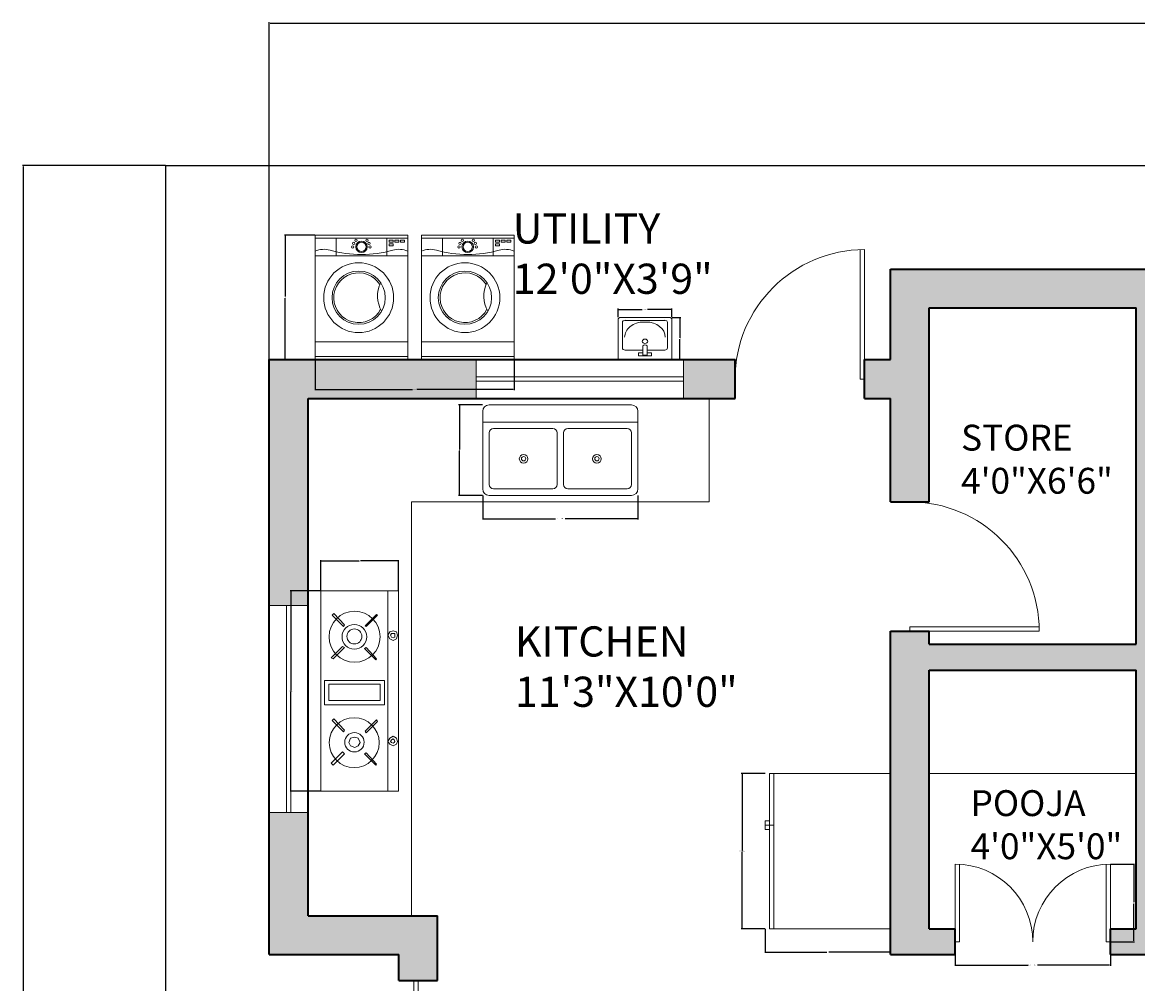
# Model space of a CAD drawing. Units: inches. Extents: x 3386 to 4477, y 1118 to 1824.
# Tile 3 of 7: x 3386 to 3645, y 1601 to 1824. Entities that reach past the tile are written whole.
import ezdxf

# ---------------------------------------------------------------- set-up
doc = ezdxf.new("R2010")
doc.units = ezdxf.units.IN
for name, color, linetype, lineweight in [('A-ANNO-DIMS', 2, 'Continuous', 18), ('A-AREA-IDEN', 7, 'Continuous', 18), ('A-DOOR', 4, 'Continuous', 18), ('A-EQPM', 9, 'Continuous', 18), ('A-FLOR-CASE', 7, 'Continuous', 18), ('A-GLAZ', 4, 'Continuous', 18), ('A-WALL', 7, 'Continuous', 35), ('C-PROP', 7, 'Continuous', 25), ('Сантехника', 7, 'Continuous', 18)]:
    doc.layers.add(name, color=color, linetype=linetype, lineweight=lineweight)
doc.layers.add('A-WALL-PATT', color=18, linetype='Continuous', lineweight=13, true_color=0x000000)
doc.styles.get("Standard").update_dxf_attribs({"font": 'arial.ttf'})
doc.dimstyles.get("Standard").update_dxf_attribs({"dimtxt": 0.18, "dimasz": 0.18, "dimexe": 0.18, "dimexo": 0.0625, "dimgap": 0.09, "dimtad": 0, "dimtih": 1, "dimtoh": 1, "dimdec": 4, "dimzin": 0, "dimdsep": 46, "dimtxsty": 'Standard', "dimcen": 0.09, "dimadec": 0, "dimazin": 0, "dimtfac": 1, "dimtdec": 4, "dimtofl": 0, "dimtmove": 0, "dimatfit": 3, "dimfxl": 1, "dimtolj": 1, "dimtzin": 0, "dimarcsym": 0})

# ---------------------------------------------------------------- blocks, each defined once
blk = doc.blocks.new('D2')
for p, q in [((0, 30), (0, 0)), ((1, 30), (1, 0)), ((0, 0), (1, 0))]:
    blk.add_line(p, q)
blk.add_arc((0, 0), 30, 0, 90)
blk = doc.blocks.new('D3')
for p, q in [((0, 0), (0, 18)), ((1, 0), (1, 18)), ((35, 0), (35, 18)), ((36, 0), (36, 18)), ((0, 0), (1, 0)), ((36, 0), (35, 0))]:
    blk.add_line(p, q)
for centre, start, end in [((0, 0), 0, 90), ((36, 0), 90, 180)]:
    blk.add_arc(centre, 18, start, end)
blk = doc.blocks.new('wash')
at = {"layer": 'Сантехника'}
for p, q in [((4817.13, 2840.92), (4788.24, 2840.92)), ((4788.24, 2819.46), (4788.24, 2840.92)), ((4788.93, 2819.46), (4788.93, 2840.92)), ((4793.08, 2819.46), (4793.08, 2840.92)), ((4812.98, 2819.46), (4812.98, 2840.92)), ((4816.44, 2819.46), (4816.44, 2840.92)), ((4817.13, 2819.46), (4817.13, 2840.92)), ((4793.08, 2836.07), (4788.93, 2836.07)), ((4793.08, 2824.31), (4788.93, 2824.31)), ((4817.13, 2819.46), (4788.24, 2819.46)), ((4817.13, 2816.27), (4788.24, 2816.27)), ((4788.24, 2794.82), (4788.24, 2816.27)), ((4788.93, 2794.82), (4788.93, 2816.27)), ((4793.08, 2794.82), (4793.08, 2816.27)), ((4812.98, 2794.82), (4812.98, 2816.27)), ((4816.44, 2794.82), (4816.44, 2816.27)), ((4817.13, 2794.82), (4817.13, 2816.27)), ((4793.08, 2811.43), (4788.93, 2811.43)), ((4793.08, 2799.66), (4788.93, 2799.66)), ((4817.13, 2794.82), (4788.24, 2794.82))]:
    blk.add_line(p, q, dxfattribs=at)
for points in [[(4789.4, 2839.27), (4789.4, 2840.17), (4789.9, 2840.17), (4789.9, 2839.27)], [(4789.4, 2837.95), (4789.4, 2838.85), (4789.9, 2838.85), (4789.9, 2837.95)], [(4789.4, 2836.64), (4789.4, 2837.53), (4789.9, 2837.53), (4789.9, 2836.64)], [(4790.27, 2836.64), (4790.27, 2837.53), (4790.77, 2837.53), (4790.77, 2836.64)], [(4789.4, 2814.62), (4789.4, 2815.52), (4789.9, 2815.52), (4789.9, 2814.62)], [(4789.4, 2813.31), (4789.4, 2814.2), (4789.9, 2814.2), (4789.9, 2813.31)], [(4789.4, 2811.99), (4789.4, 2812.89), (4789.9, 2812.89), (4789.9, 2811.99)], [(4790.27, 2811.99), (4790.27, 2812.89), (4790.77, 2812.89), (4790.77, 2811.99)]]:
    blk.add_lwpolyline(points, close=True, dxfattribs=at)
for centre, radius in [((4802.77, 2829.54), 8.1), ((4802.77, 2829.54), 6.17), ((4789.46, 2831.45), 0.271), ((4790.19, 2831.93), 0.271), ((4790.98, 2832.18), 0.271), ((4789.46, 2828.92), 0.271), ((4790.98, 2830.19), 1.34), ((4790.98, 2830.19), 1.07), ((4790.19, 2828.4), 0.271), ((4790.98, 2828.15), 0.271), ((4802.77, 2804.9), 8.1), ((4802.77, 2804.9), 6.17), ((4789.46, 2806.8), 0.271), ((4790.98, 2805.55), 1.34), ((4790.19, 2807.28), 0.271), ((4790.98, 2805.55), 1.07), ((4790.98, 2807.53), 0.271), ((4789.46, 2804.27), 0.271), ((4790.19, 2803.75), 0.271), ((4790.98, 2803.5), 0.271)]:
    blk.add_circle(centre, radius, dxfattribs=at)
for centre, radius, start, end in [((4796.44, 2838.85), 4.89, 154.895, 196.6068), ((4762.87, 2829.66), 29.92, 1.0206, 15.0937), ((4802.77, 2829.54), 5.77, 121.8067, 62.1506), ((4802.39, 2840.74), 6.83, 243.19, 300.7673), ((4762.87, 2830.72), 29.92, 344.9063, 358.9794), ((4796.44, 2821.54), 4.89, 163.3932, 205.105), ((4796.44, 2814.2), 4.89, 154.895, 196.6068), ((4762.87, 2805.01), 29.92, 1.0206, 15.0937), ((4802.77, 2804.9), 5.77, 121.8067, 62.1506), ((4802.39, 2816.1), 6.83, 243.19, 300.7673), ((4762.87, 2806.08), 29.92, 344.9063, 358.9794), ((4796.44, 2796.89), 4.89, 163.3932, 205.105)]:
    blk.add_arc(centre, radius, start, end, dxfattribs=at)
blk = doc.blocks.new('Rac7')
at = {"color": 0}
for p, q in [((-39501, -24232), (-39501, -23830)), ((-39474, -23808), (-38988, -23808)), ((-38961, -23830), (-38961, -24232)), ((-39457, -23859), (-39457, -24115)), ((-39032, -23838), (-39430, -23838)), ((-39221, -23855), (-39241, -23855)), ((-39005, -24115), (-39005, -23859)), ((-39005, -23859), (-39005, -23859)), ((-39430, -24136), (-39253, -24136)), ((-39297, -24164), (-39253, -24164)), ((-39297, -24194), (-39297, -24164)), ((-39253, -24186), (-39253, -24094)), ((-39209, -24186), (-39209, -24094)), ((-39209, -24136), (-39032, -24136)), ((-39209, -24164), (-39165, -24164)), ((-39165, -24164), (-39165, -24194)), ((-38961, -24232), (-39501, -24232)), ((-39165, -24194), (-39297, -24194)), ((-39253, -24186), (-39209, -24186))]:
    blk.add_line(p, q, dxfattribs=at)
at = {"color": 0, "extrusion": (0, 0, -1)}
for centre, major_axis, start_param, end_param in [((-39474, -23830), (-27, 0), 0, 1.570796), ((-38988, -23830), (-27, 0), 1.570796, 3.141593), ((-39430, -23859), (-27, 0), 0, 1.570796), ((-39241, -24007), (-194, 0), 0, 1.570796), ((-39221, -24007), (-194, 0), 1.570796, 3.141593), ((-39032, -23859), (-27, 0), 1.570796, 3.141593), ((-39430, -24115), (-27, 0), -1.570796, 0), ((-39231, -24104), (-25.3, 0), 0.552816, 2.588777), ((-39032, -24115), (-27, 0), -3.141593, -1.570796)]:
    blk.add_ellipse(centre, major_axis=major_axis, ratio=0.785714, start_param=start_param, end_param=end_param, dxfattribs=at)
blk.add_ellipse((-39231, -24048), major_axis=(-27.9, 0), ratio=0.785714, dxfattribs=at)
blk = doc.blocks.new('Sink-double - 36 in top')
for p, q in [((-18, -4), (18, -4)), ((-0.75, -18.5), (-0.75, -6.5)), ((0.75, -6.5), (0.75, -18.5))]:
    blk.add_line(p, q)
for points in [[(-16.5, 0), (16.5, 0)], [(-18, -19.5), (-18, -1.5)], [(18, -1.5), (18, -19.5)], [(-16.5, -18.5), (-16.5, -6.5)], [(-15.5, -5.5), (-1.75, -5.5)], [(1.75, -5.5), (15.5, -5.5)], [(16.5, -6.5), (16.5, -18.5)], [(-1.75, -19.5), (-15.5, -19.5)], [(15.5, -19.5), (1.75, -19.5)], [(16.5, -21), (-16.5, -21)]]:
    blk.add_lwpolyline(points)
for centre, radius in [((-8.5, -12.5), 1), ((-8.5, -12.5), 0.5), ((8.5, -12.5), 1), ((8.5, -12.5), 0.5)]:
    blk.add_circle(centre, radius)
for centre, radius, start, end in [((-16.5, -1.5), 1.5, 90, 180), ((16.5, -1.5), 1.5, 0, 90), ((-15.5, -6.5), 1, 90, 180), ((-1.75, -6.5), 1, 0, 90), ((1.75, -6.5), 1, 90, 180), ((15.5, -6.5), 1, 0, 90), ((-16.5, -19.5), 1.5, 180, 270), ((-15.5, -18.5), 1, 180, 270), ((-1.75, -18.5), 1, 270, 0), ((1.75, -18.5), 1, 180, 270), ((15.5, -18.5), 1, 270, 0), ((16.5, -19.5), 1.5, 270, 0)]:
    blk.add_arc(centre, radius, start, end)
blk = doc.blocks.new('gas 1')
for points in [[(35.93, -1.87), (35.93, 0), (0, 0), (0, -1.87)], [(8.12, -0.94), (8.44, -1.56), (8.91, -1.87), (9.53, -1.56), (9.84, -0.94), (9.53, -0.31), (8.91, -0.16), (8.44, -0.31)], [(8.59, -0.94), (8.75, -1.25), (8.91, -1.41), (9.22, -1.25), (9.37, -0.94), (9.22, -0.78), (8.91, -0.62), (8.75, -0.78)], [(27.03, -0.94), (27.34, -1.56), (27.97, -1.87), (28.59, -1.56), (28.75, -0.94), (28.59, -0.31), (27.97, -0.16), (27.34, -0.31)], [(27.5, -0.94), (27.65, -1.25), (27.97, -1.41), (28.28, -1.25), (28.28, -0.94), (28.28, -0.62), (27.97, -0.62), (27.65, -0.62)], [(4.84, -3.91), (4.69, -4.06), (6.72, -6.09), (6.87, -5.78)], [(12.81, -3.91), (12.5, -3.75), (10.47, -5.78), (10.78, -5.94)], [(19.84, -13.28), (15.47, -13.28), (15.47, -2.5), (19.84, -2.5)], [(19.22, -12.5), (16.25, -12.5), (16.25, -3.28), (19.22, -3.28)], [(23.75, -3.91), (23.59, -4.06), (25.62, -6.09), (25.78, -5.78)], [(31.71, -3.91), (31.56, -3.75), (29.53, -5.78), (29.68, -5.94)], [(7.81, -7.81), (8.12, -8.59), (8.75, -8.91), (9.53, -8.59), (9.69, -7.81), (9.53, -7.19), (8.75, -6.87), (8.12, -7.19)], [(7.03, -10), (6.72, -9.69), (4.69, -11.72), (5, -12.03)], [(12.97, -11.56), (10.94, -9.69), (10.62, -9.84), (12.65, -11.87)], [(23.75, -11.72), (23.9, -12.03), (25.93, -10), (25.78, -9.69)], [(31.87, -11.56), (29.84, -9.69), (29.53, -9.84), (31.56, -11.87)]]:
    blk.add_lwpolyline(points, close=True)
blk.add_lwpolyline([(35.93, -1.87), (35.93, -13.9), (0, -13.9), (0, -1.87)])
for centre, radius in [((8.7, -7.92), 4.48), ((27.7, -7.86), 4.58), ((27.69, -7.89), 2.22), ((8.77, -7.89), 1.74), ((27.76, -7.89), 1.35)]:
    blk.add_circle(centre, radius)
blk = doc.blocks.new('Refrigerator-2 door - 36 in top')
for p, q in [((0, -26.999999), (36, -26.999999)), ((11, -27.999999), (11, -28.999999)), ((12, -26.999999), (12, -28.999999)), ((13, -28.999999), (13, -27.999999)), ((11, -28.999999), (13, -28.999999))]:
    blk.add_line(p, q)
blk.add_lwpolyline([(0, -27.999999), (0, 0), (36, 0), (36, -27.999999)], close=True)
blk = doc.blocks.new('WIN-48IN')
for p, q in [((0, 48), (9, 48)), ((4, 0), (4, 48)), ((5, 0), (5, 48)), ((0, 0), (9, 0))]:
    blk.add_line(p, q)
blk = doc.blocks.new('DOOR-SLIDING-84IN')
for p, q in [((0, 42), (0, 84)), ((1, 84), (1, 0)), ((1, 42), (0, 42)), ((1, 42), (2, 42)), ((2, 42), (2, 0))]:
    blk.add_line(p, q)
blk = doc.blocks.new('*D69')
at = {"layer": 'A-ANNO-DIMS', "color": 0, "lineweight": -2, "transparency": 16777216}
for p, q in [((3602.66, 1610.81), (3602.66, 1605.29)), ((3638.66, 1610.81), (3638.66, 1605.29)), ((3602.84, 1605.47), (3619.57, 1605.47)), ((3638.48, 1605.47), (3621.74, 1605.47))]:
    blk.add_line(p, q, dxfattribs=at)
at = {"layer": 'A-ANNO-DIMS', "color": 0, "transparency": 16777216}
for points in [[(3602.84, 1605.5), (3602.84, 1605.44), (3602.66, 1605.47)], [(3638.48, 1605.5), (3638.48, 1605.44), (3638.66, 1605.47)]]:
    blk.add_solid(points, dxfattribs=at)
at = {"layer": 'Defpoints', "color": 0, "transparency": 16777216}
for p in [(3602.66, 1610.87), (3638.66, 1610.87), (3638.66, 1605.47)]:
    blk.add_point(p, dxfattribs=at)
at = {"layer": 'A-ANNO-DIMS', "color": 0, "transparency": 16777216, "insert": (3620.66, 1605.47), "char_height": 0.18, "attachment_point": 5}
blk.add_mtext('\\A1;POOJA DOOR 36', dxfattribs=at)
blk = doc.blocks.new('*D70')
at = {"layer": 'A-ANNO-DIMS', "color": 0, "lineweight": -2, "transparency": 16777216}
for p, q in [((3638.72, 1628.87), (3644.24, 1628.87)), ((3644.06, 1628.69), (3644.06, 1620.05)), ((3644.06, 1611.05), (3644.06, 1619.69)), ((3638.72, 1610.87), (3644.24, 1610.87))]:
    blk.add_line(p, q, dxfattribs=at)
at = {"layer": 'A-ANNO-DIMS', "color": 0, "transparency": 16777216}
for points in [[(3644.03, 1628.69), (3644.09, 1628.69), (3644.06, 1628.87)], [(3644.03, 1611.05), (3644.09, 1611.05), (3644.06, 1610.87)]]:
    blk.add_solid(points, dxfattribs=at)
at = {"layer": 'Defpoints', "color": 0, "transparency": 16777216}
for p in [(3638.66, 1628.87), (3644.06, 1628.87), (3638.66, 1610.87)]:
    blk.add_point(p, dxfattribs=at)
at = {"layer": 'A-ANNO-DIMS', "color": 0, "transparency": 16777216, "insert": (3644.06, 1619.87), "char_height": 0.18, "attachment_point": 5}
blk.add_mtext('\\A1;18', dxfattribs=at)
blk = doc.blocks.new('*D87')
at = {"layer": 'A-ANNO-DIMS', "color": 0, "lineweight": -2, "transparency": 16777216}
for p, q in [((3454.3, 1745.81), (3454.3, 1738.77)), ((3500.4, 1745.81), (3500.4, 1738.77)), ((3454.48, 1738.95), (3476.85, 1738.95)), ((3500.22, 1738.95), (3477.85, 1738.95))]:
    blk.add_line(p, q, dxfattribs=at)
at = {"layer": 'A-ANNO-DIMS', "color": 0, "transparency": 16777216}
for points in [[(3454.48, 1738.98), (3454.48, 1738.92), (3454.3, 1738.95)], [(3500.22, 1738.98), (3500.22, 1738.92), (3500.4, 1738.95)]]:
    blk.add_solid(points, dxfattribs=at)
at = {"layer": 'Defpoints', "color": 0, "transparency": 16777216}
for p in [(3454.3, 1745.87), (3500.4, 1745.87), (3500.4, 1738.95)]:
    blk.add_point(p, dxfattribs=at)
at = {"layer": 'A-ANNO-DIMS', "color": 0, "transparency": 16777216, "insert": (3477.35, 1738.95), "char_height": 0.18, "attachment_point": 5}
blk.add_mtext('\\A1;W/D 46', dxfattribs=at)
blk = doc.blocks.new('*D88')
at = {"layer": 'A-ANNO-DIMS', "color": 0, "lineweight": -2, "transparency": 16777216}
for p, q in [((3454.24, 1774.76), (3447.2, 1774.76)), ((3447.38, 1774.58), (3447.38, 1760.5)), ((3447.38, 1746.05), (3447.38, 1760.13)), ((3454.24, 1745.87), (3447.2, 1745.87))]:
    blk.add_line(p, q, dxfattribs=at)
at = {"layer": 'A-ANNO-DIMS', "color": 0, "transparency": 16777216}
for points in [[(3447.35, 1774.58), (3447.41, 1774.58), (3447.38, 1774.76)], [(3447.35, 1746.05), (3447.41, 1746.05), (3447.38, 1745.87)]]:
    blk.add_solid(points, dxfattribs=at)
at = {"layer": 'Defpoints', "color": 0, "transparency": 16777216}
for p in [(3454.3, 1774.76), (3447.38, 1745.87), (3454.3, 1745.87)]:
    blk.add_point(p, dxfattribs=at)
at = {"layer": 'A-ANNO-DIMS', "color": 0, "transparency": 16777216, "insert": (3447.38, 1760.32), "char_height": 0.18, "attachment_point": 5}
blk.add_mtext('\\A1;29', dxfattribs=at)
blk = doc.blocks.new('*D89')
at = {"layer": 'A-ANNO-DIMS', "color": 0, "lineweight": -2, "transparency": 16777216}
for p, q in [((3524.53, 1755.72), (3524.53, 1757.71)), ((3524.71, 1757.53), (3530.13, 1757.53)), ((3536.81, 1757.53), (3531.38, 1757.53)), ((3536.99, 1755.72), (3536.99, 1757.71))]:
    blk.add_line(p, q, dxfattribs=at)
at = {"layer": 'A-ANNO-DIMS', "color": 0, "transparency": 16777216}
for points in [[(3524.71, 1757.56), (3524.71, 1757.5), (3524.53, 1757.53)], [(3536.81, 1757.56), (3536.81, 1757.5), (3536.99, 1757.53)]]:
    blk.add_solid(points, dxfattribs=at)
at = {"layer": 'Defpoints', "color": 0, "transparency": 16777216}
for p in [(3524.53, 1757.53), (3524.53, 1755.66), (3536.99, 1755.66)]:
    blk.add_point(p, dxfattribs=at)
at = {"layer": 'A-ANNO-DIMS', "color": 0, "transparency": 16777216, "insert": (3530.76, 1757.53), "char_height": 0.18, "attachment_point": 5}
blk.add_mtext('\\A1;BASIN 12', dxfattribs=at)
blk = doc.blocks.new('*D90')
at = {"layer": 'A-ANNO-DIMS', "color": 0, "lineweight": -2, "transparency": 16777216}
for p, q in [((3537.05, 1755.66), (3539.04, 1755.66)), ((3538.86, 1755.48), (3538.86, 1750.95)), ((3538.86, 1746.05), (3538.86, 1750.58)), ((3537.05, 1745.87), (3539.04, 1745.87))]:
    blk.add_line(p, q, dxfattribs=at)
at = {"layer": 'A-ANNO-DIMS', "color": 0, "transparency": 16777216}
for points in [[(3538.83, 1755.48), (3538.89, 1755.48), (3538.86, 1755.66)], [(3538.83, 1746.05), (3538.89, 1746.05), (3538.86, 1745.87)]]:
    blk.add_solid(points, dxfattribs=at)
at = {"layer": 'Defpoints', "color": 0, "transparency": 16777216}
for p in [(3536.99, 1755.66), (3538.86, 1755.66), (3536.99, 1745.87)]:
    blk.add_point(p, dxfattribs=at)
at = {"layer": 'A-ANNO-DIMS', "color": 0, "transparency": 16777216, "insert": (3538.86, 1750.76), "char_height": 0.18, "attachment_point": 5}
blk.add_mtext('\\A1;10', dxfattribs=at)
blk = doc.blocks.new('*D95')
at = {"layer": 'A-ANNO-DIMS', "color": 0, "lineweight": -2, "transparency": 16777216}
for p, q in [((3493.13, 1714.32), (3493.13, 1708.8)), ((3529.13, 1714.32), (3529.13, 1708.8)), ((3493.31, 1708.98), (3510.04, 1708.98)), ((3528.95, 1708.98), (3512.23, 1708.98))]:
    blk.add_line(p, q, dxfattribs=at)
at = {"layer": 'A-ANNO-DIMS', "color": 0, "transparency": 16777216}
for points in [[(3493.31, 1709.01), (3493.31, 1708.95), (3493.13, 1708.98)], [(3528.95, 1709.01), (3528.95, 1708.95), (3529.13, 1708.98)]]:
    blk.add_solid(points, dxfattribs=at)
at = {"layer": 'Defpoints', "color": 0, "transparency": 16777216}
for p in [(3493.13, 1714.38), (3529.13, 1714.38), (3493.13, 1708.98)]:
    blk.add_point(p, dxfattribs=at)
at = {"layer": 'A-ANNO-DIMS', "color": 0, "transparency": 16777216, "insert": (3511.13, 1708.98), "char_height": 0.18, "attachment_point": 5}
blk.add_mtext('\\A1;DOUBLE SINK 36', dxfattribs=at)
blk = doc.blocks.new('*D96')
at = {"layer": 'A-ANNO-DIMS', "color": 0, "lineweight": -2, "transparency": 16777216}
for p, q in [((3493.07, 1735.38), (3487.55, 1735.38)), ((3487.73, 1735.2), (3487.73, 1725.06)), ((3487.73, 1714.56), (3487.73, 1724.7)), ((3493.07, 1714.38), (3487.55, 1714.38))]:
    blk.add_line(p, q, dxfattribs=at)
at = {"layer": 'A-ANNO-DIMS', "color": 0, "transparency": 16777216}
for points in [[(3487.7, 1735.2), (3487.76, 1735.2), (3487.73, 1735.38)], [(3487.7, 1714.56), (3487.76, 1714.56), (3487.73, 1714.38)]]:
    blk.add_solid(points, dxfattribs=at)
at = {"layer": 'Defpoints', "color": 0, "transparency": 16777216}
for p in [(3487.73, 1735.38), (3493.13, 1735.38), (3493.13, 1714.38)]:
    blk.add_point(p, dxfattribs=at)
at = {"layer": 'A-ANNO-DIMS', "color": 0, "transparency": 16777216, "insert": (3487.73, 1724.88), "char_height": 0.18, "attachment_point": 5}
blk.add_mtext('\\A1;21', dxfattribs=at)
blk = doc.blocks.new('*D97')
at = {"layer": 'A-ANNO-DIMS', "color": 0, "lineweight": -2, "transparency": 16777216}
for p, q in [((3455.55, 1692.24), (3448.47, 1692.24)), ((3448.65, 1692.06), (3448.65, 1669.2)), ((3448.65, 1645.97), (3448.65, 1668.83)), ((3455.55, 1645.79), (3448.47, 1645.79))]:
    blk.add_line(p, q, dxfattribs=at)
at = {"layer": 'A-ANNO-DIMS', "color": 0, "transparency": 16777216}
for points in [[(3448.62, 1692.06), (3448.68, 1692.06), (3448.65, 1692.24)], [(3448.62, 1645.97), (3448.68, 1645.97), (3448.65, 1645.79)]]:
    blk.add_solid(points, dxfattribs=at)
at = {"layer": 'Defpoints', "color": 0, "transparency": 16777216}
for p in [(3448.65, 1692.24), (3455.61, 1692.24), (3455.61, 1645.79)]:
    blk.add_point(p, dxfattribs=at)
at = {"layer": 'A-ANNO-DIMS', "color": 0, "transparency": 16777216, "insert": (3448.65, 1669.01), "char_height": 0.18, "attachment_point": 5}
blk.add_mtext('\\A1;HOB 46', dxfattribs=at)
blk = doc.blocks.new('*D98')
at = {"layer": 'A-ANNO-DIMS', "color": 0, "lineweight": -2, "transparency": 16777216}
for p, q in [((3455.61, 1692.3), (3455.61, 1699.38)), ((3455.79, 1699.2), (3464.39, 1699.2)), ((3473.41, 1699.2), (3464.81, 1699.2)), ((3473.59, 1692.3), (3473.59, 1699.38))]:
    blk.add_line(p, q, dxfattribs=at)
at = {"layer": 'A-ANNO-DIMS', "color": 0, "transparency": 16777216}
for points in [[(3455.79, 1699.23), (3455.79, 1699.17), (3455.61, 1699.2)], [(3473.41, 1699.23), (3473.41, 1699.17), (3473.59, 1699.2)]]:
    blk.add_solid(points, dxfattribs=at)
at = {"layer": 'Defpoints', "color": 0, "transparency": 16777216}
for p in [(3473.59, 1699.2), (3455.61, 1692.24), (3473.59, 1692.24)]:
    blk.add_point(p, dxfattribs=at)
at = {"layer": 'A-ANNO-DIMS', "color": 0, "transparency": 16777216, "insert": (3464.6, 1699.2), "char_height": 0.18, "attachment_point": 5}
blk.add_mtext('\\A1;18', dxfattribs=at)
blk = doc.blocks.new('*D99')
at = {"layer": 'A-ANNO-DIMS', "color": 0, "lineweight": -2, "transparency": 16777216}
for p, q in [((3558.59, 1649.87), (3553.08, 1649.87)), ((3553.26, 1649.69), (3553.26, 1632.05)), ((3553.26, 1614.05), (3553.26, 1631.68)), ((3558.59, 1613.87), (3553.08, 1613.87))]:
    blk.add_line(p, q, dxfattribs=at)
at = {"layer": 'A-ANNO-DIMS', "color": 0, "transparency": 16777216}
for points in [[(3553.23, 1649.69), (3553.29, 1649.69), (3553.26, 1649.87)], [(3553.23, 1614.05), (3553.29, 1614.05), (3553.26, 1613.87)]]:
    blk.add_solid(points, dxfattribs=at)
at = {"layer": 'Defpoints', "color": 0, "transparency": 16777216}
for p in [(3558.66, 1649.87), (3553.26, 1613.87), (3558.66, 1613.87)]:
    blk.add_point(p, dxfattribs=at)
at = {"layer": 'A-ANNO-DIMS', "color": 0, "transparency": 16777216, "insert": (3553.26, 1631.87), "char_height": 0.18, "attachment_point": 5}
blk.add_mtext('\\A1;FRIDGE 36', dxfattribs=at)
blk = doc.blocks.new('*D100')
at = {"layer": 'A-ANNO-DIMS', "color": 0, "lineweight": -2, "transparency": 16777216}
for p, q in [((3558.66, 1613.81), (3558.66, 1608.29)), ((3587.66, 1613.81), (3587.66, 1608.29)), ((3558.84, 1608.47), (3572.93, 1608.47)), ((3587.48, 1608.47), (3573.38, 1608.47))]:
    blk.add_line(p, q, dxfattribs=at)
at = {"layer": 'A-ANNO-DIMS', "color": 0, "transparency": 16777216}
for points in [[(3558.84, 1608.5), (3558.84, 1608.44), (3558.66, 1608.47)], [(3587.48, 1608.5), (3587.48, 1608.44), (3587.66, 1608.47)]]:
    blk.add_solid(points, dxfattribs=at)
at = {"layer": 'Defpoints', "color": 0, "transparency": 16777216}
for p in [(3558.66, 1613.87), (3587.66, 1613.87), (3587.66, 1608.47)]:
    blk.add_point(p, dxfattribs=at)
at = {"layer": 'A-ANNO-DIMS', "color": 0, "transparency": 16777216, "insert": (3573.16, 1608.47), "char_height": 0.18, "attachment_point": 5}
blk.add_mtext('\\A1;29', dxfattribs=at)
blk = doc.blocks.new('*D102')
at = {"layer": 'A-ANNO-DIMS', "color": 0, "lineweight": -2, "transparency": 16777216}
for p, q in [((3419.59, 1790.87), (3386.43, 1790.87)), ((3386.61, 1790.69), (3386.61, 1491.05)), ((3386.61, 1191.05), (3386.61, 1490.69)), ((3419.59, 1190.87), (3386.43, 1190.87))]:
    blk.add_line(p, q, dxfattribs=at)
at = {"layer": 'A-ANNO-DIMS', "color": 0, "transparency": 16777216}
for points in [[(3386.58, 1790.69), (3386.64, 1790.69), (3386.61, 1790.87)], [(3386.58, 1191.05), (3386.64, 1191.05), (3386.61, 1190.87)]]:
    blk.add_solid(points, dxfattribs=at)
at = {"layer": 'Defpoints', "color": 0, "transparency": 16777216}
for p in [(3386.61, 1790.87), (3419.66, 1790.87), (3419.66, 1190.87)]:
    blk.add_point(p, dxfattribs=at)
at = {"layer": 'A-ANNO-DIMS', "color": 0, "transparency": 16777216, "insert": (3386.61, 1490.87), "char_height": 0.18, "attachment_point": 5}
blk.add_mtext('\\A1;600', dxfattribs=at)
blk = doc.blocks.new('*D103')
at = {"layer": 'A-ANNO-DIMS', "color": 0, "lineweight": -2, "transparency": 16777216}
for p, q in [((3443.66, 1745.93), (3443.66, 1824.1)), ((3443.84, 1823.92), (3659.36, 1823.92)), ((3875.48, 1823.92), (3659.95, 1823.92)), ((3875.66, 1766.93), (3875.66, 1824.1))]:
    blk.add_line(p, q, dxfattribs=at)
at = {"layer": 'A-ANNO-DIMS', "color": 0, "transparency": 16777216}
for points in [[(3443.84, 1823.95), (3443.84, 1823.89), (3443.66, 1823.92)], [(3875.48, 1823.95), (3875.48, 1823.89), (3875.66, 1823.92)]]:
    blk.add_solid(points, dxfattribs=at)
at = {"layer": 'Defpoints', "color": 0, "transparency": 16777216}
for p in [(3875.66, 1823.92), (3875.66, 1766.87), (3443.66, 1745.87)]:
    blk.add_point(p, dxfattribs=at)
at = {"layer": 'A-ANNO-DIMS', "color": 0, "transparency": 16777216, "insert": (3659.66, 1823.92), "char_height": 0.18, "attachment_point": 5}
blk.add_mtext('\\A1;432', dxfattribs=at)

msp = doc.modelspace()

# ---------------------------------------------------------------- hatches: boundary and pattern name
at = {"layer": 'A-WALL-PATT'}
h = msp.add_hatch(color=256, dxfattribs=at)
h.dxf.hatch_style = 1
h.paths.add_polyline_path([(3443.66, 1221.87), (3452.66, 1221.87), (3452.66, 1301.87), (3458.66, 1301.87), (3458.66, 1310.87), (3452.66, 1310.87), (3452.66, 1328.87), (3443.66, 1328.87)])
h.paths.add_polyline_path([(3506.66, 1310.87), (3506.66, 1306.37), (3506.66, 1301.87), (3530.66, 1301.87), (3530.66, 1310.87)])
h.paths.add_polyline_path([(3653.66, 1301.87), (3653.66, 1382.87), (3662.66, 1382.87), (3662.66, 1391.87), (3653.66, 1391.87), (3653.66, 1529.87), (3659.66, 1529.87), (3659.66, 1535.87), (3644.66, 1535.87), (3644.66, 1310.87), (3602.66, 1310.87), (3602.66, 1301.87)])
h.paths.add_polyline_path([(3452.66, 1406.87), (3443.66, 1406.87), (3443.66, 1376.87), (3452.66, 1376.87), (3452.66, 1388.44)])
h.paths.add_polyline_path([(3452.66, 1478.87), (3452.66, 1502.87), (3478.74, 1502.87), (3482.66, 1502.87), (3482.66, 1504.87), (3482.66, 1517.87), (3473.66, 1517.87), (3473.66, 1511.87), (3443.66, 1511.87), (3443.66, 1478.87)])
h.paths.add_polyline_path([(3773.66, 1391.87), (3710.66, 1391.87), (3710.66, 1382.87), (3773.66, 1382.87)], flags=17)
h.paths.add_polyline_path([(3824.66, 1391.87), (3806.66, 1391.87), (3806.66, 1469.87), (3809.66, 1469.87), (3809.66, 1472.87), (3809.66, 1475.87), (3806.66, 1475.87), (3806.66, 1478.87), (3800.66, 1478.87), (3800.66, 1463.32), (3800.66, 1391.87), (3797.66, 1391.87), (3797.66, 1382.87), (3824.66, 1382.87)], flags=17)
h.paths.add_polyline_path([(3866.66, 1469.87), (3866.66, 1391.87), (3848.66, 1391.87), (3848.66, 1382.87), (3875.66, 1382.87), (3875.66, 1547.87), (3866.66, 1547.87), (3866.66, 1535.87), (3695.66, 1535.87), (3695.66, 1529.87), (3800.66, 1529.87), (3800.66, 1508.87), (3806.66, 1508.87), (3806.66, 1529.87), (3866.66, 1529.87), (3866.66, 1475.87), (3839.66, 1475.87), (3839.66, 1469.87)])
h.paths.add_polyline_path([(3875.66, 1673.87), (3866.66, 1673.87), (3866.66, 1663.37), (3866.66, 1647.44), (3866.66, 1613.87), (3761.66, 1613.87), (3761.66, 1607.87), (3866.66, 1607.87), (3866.66, 1595.87), (3875.66, 1595.87)])
h.paths.add_polyline_path([(3473.66, 1607.87), (3473.66, 1601.87), (3482.66, 1601.87), (3482.66, 1616.87), (3452.66, 1616.87), (3452.66, 1640.87), (3443.66, 1640.87), (3443.66, 1607.87)])
h.paths.add_polyline_path([(3491.66, 1736.87), (3491.66, 1745.87), (3478.95, 1745.87), (3443.66, 1745.87), (3443.66, 1688.87), (3452.66, 1688.87), (3452.66, 1736.87)])
h.paths.add_polyline_path([(3551.66, 1745.87), (3539.66, 1745.87), (3539.66, 1736.87), (3551.66, 1736.87)])
h.paths.add_polyline_path([(3587.66, 1745.87), (3581.66, 1745.87), (3581.66, 1741.37), (3581.66, 1736.87), (3587.66, 1736.87), (3587.66, 1712.87), (3596.66, 1712.87), (3596.66, 1757.87), (3644.66, 1757.87), (3644.66, 1679.87), (3596.66, 1679.87), (3596.66, 1682.87), (3592.16, 1682.87), (3587.66, 1682.87), (3587.66, 1607.87), (3602.66, 1607.87), (3602.66, 1613.87), (3596.66, 1613.87), (3596.66, 1673.87), (3644.66, 1673.87), (3644.66, 1613.87), (3638.66, 1613.87), (3638.66, 1610.87), (3638.66, 1607.87), (3725.66, 1607.87), (3725.66, 1613.87), (3722.66, 1613.87), (3722.66, 1634.87), (3716.66, 1634.87), (3716.66, 1613.87), (3650.66, 1613.87), (3650.66, 1673.87), (3683.66, 1673.87), (3683.66, 1679.87), (3650.66, 1679.87), (3650.66, 1757.87), (3671.66, 1757.87), (3671.66, 1766.87), (3587.66, 1766.87)])
h.paths.add_polyline_path([(3716.66, 1757.87), (3716.66, 1679.87), (3713.66, 1679.87), (3713.66, 1673.87), (3716.66, 1673.87), (3716.66, 1664.87), (3722.66, 1664.87), (3722.66, 1757.87), (3728.66, 1757.87), (3728.66, 1766.87), (3695.66, 1766.87), (3695.66, 1757.87)])
h.paths.add_polyline_path([(3806.66, 1757.87), (3806.66, 1766.87), (3776.66, 1766.87), (3776.66, 1757.87)])
h.paths.add_polyline_path([(3875.66, 1766.87), (3854.66, 1766.87), (3854.66, 1757.87), (3866.66, 1757.87), (3866.66, 1733.87), (3875.66, 1733.87)])

# ---------------------------------------------------------------- linework, layer by layer
at = {"layer": 'A-FLOR-CASE'}
for p, q in [((3545.66, 1736.87), (3545.66, 1712.87)), ((3476.66, 1616.87), (3476.66, 1712.87)), ((3476.66, 1712.87), (3545.66, 1712.87)), ((3596.66, 1649.87), (3644.66, 1649.87))]:
    msp.add_line(p, q, dxfattribs=at)
at = {"layer": 'A-WALL'}
for p, q in [((3587.66, 1766.87), (3875.66, 1766.87)), ((3587.66, 1745.87), (3587.66, 1766.87)), ((3596.66, 1757.87), (3644.66, 1757.87)), ((3596.66, 1712.87), (3596.66, 1757.87)), ((3644.66, 1679.87), (3644.66, 1757.87)), ((3443.66, 1607.87), (3443.66, 1745.87)), ((3443.66, 1745.87), (3551.66, 1745.87)), ((3551.66, 1736.87), (3551.66, 1745.87)), ((3581.66, 1736.87), (3581.66, 1745.87)), ((3581.66, 1745.87), (3587.66, 1745.87)), ((3452.66, 1616.87), (3452.66, 1736.87)), ((3452.66, 1736.87), (3551.66, 1736.87)), ((3581.66, 1736.87), (3587.66, 1736.87)), ((3587.66, 1712.87), (3587.66, 1736.87)), ((3587.66, 1712.87), (3596.66, 1712.87)), ((3587.66, 1607.87), (3587.66, 1682.87)), ((3587.66, 1682.87), (3596.66, 1682.87)), ((3596.66, 1679.87), (3596.66, 1682.87)), ((3596.66, 1679.87), (3644.66, 1679.87)), ((3596.66, 1673.87), (3644.66, 1673.87)), ((3596.66, 1613.87), (3596.66, 1673.87)), ((3644.66, 1613.87), (3644.66, 1673.87)), ((3452.66, 1616.87), (3482.66, 1616.87)), ((3482.66, 1601.87), (3482.66, 1616.87)), ((3596.66, 1613.87), (3602.66, 1613.87)), ((3602.66, 1607.87), (3602.66, 1613.87)), ((3638.66, 1607.87), (3638.66, 1613.87)), ((3638.66, 1613.87), (3644.66, 1613.87)), ((3443.66, 1607.87), (3473.66, 1607.87)), ((3473.66, 1601.87), (3473.66, 1607.87)), ((3587.66, 1607.87), (3602.66, 1607.87)), ((3638.66, 1607.87), (3725.66, 1607.87)), ((3473.66, 1601.87), (3482.66, 1601.87))]:
    msp.add_line(p, q, dxfattribs=at)
at = {"layer": 'C-PROP'}
msp.add_lwpolyline([(3419.66, 1790.87), (3899.66, 1790.87), (3899.66, 1190.87), (3419.66, 1190.87)], close=True, dxfattribs=at)

# ---------------------------------------------------------------- block references
at = {"layer": 'A-DOOR', "xscale": -1}
msp.add_blockref('D2', (3581.66, 1741.37), dxfattribs=at)
at = {"layer": 'A-DOOR', "xscale": -1, "rotation": 270}
msp.add_blockref('D2', (3592.16, 1682.87), dxfattribs=at)
at = {"layer": 'A-DOOR'}
for name, p in [('D3', (3602.66, 1610.87)), ('DOOR-SLIDING-84IN', (3477.16, 1517.87))]:
    msp.add_blockref(name, p, dxfattribs=at)
at = {"layer": 'A-EQPM', "rotation": 270}
for name, p in [('wash', (659.48, 6563)), ('Refrigerator-2 door - 36 in top', (3587.66, 1649.87))]:
    msp.add_blockref(name, p, dxfattribs=at)
at = {"layer": 'A-EQPM', "xscale": -1.292580420916565, "yscale": 1.292580420916565, "zscale": 1.292580420916565, "rotation": 270}
msp.add_blockref('gas 1', (3473.59, 1645.79), dxfattribs=at)
at = {"layer": 'A-GLAZ', "rotation": 269.999999999999}
msp.add_blockref('WIN-48IN', (3491.66, 1745.87), dxfattribs=at)
at = {"layer": 'A-GLAZ'}
msp.add_blockref('WIN-48IN', (3443.66, 1640.87), dxfattribs=at)
at = {"layer": 'Сантехника', "xscale": -0.0231094998546128, "yscale": 0.0231094998546128, "zscale": 0.0231094998546128}
msp.add_blockref('Rac7', (2624.15, 2305.86), dxfattribs=at)
at = {"layer": 'Сантехника', "xscale": -1}
msp.add_blockref('Sink-double - 36 in top', (3511.13, 1735.38), dxfattribs=at)

# ---------------------------------------------------------------- texts
at = {"layer": 'A-AREA-IDEN', "attachment_point": 1}
for s, width, heights, insert, char_height in [('{\\fTimes New Roman|b0|i0|c0|p18;UTILITY\\P12\'0"X3\'9"}', 113.4175, [0], (3500.11, 1779.79), 7), ('{\\fTimes New Roman|b0|i0|c0|p18;STORE\\P4\'0"X6\'6"}', 79.5604, [0], (3604.04, 1730.77), 6), ('{\\fTimes New Roman|b0|i0|c0|p18;KITCHEN\\P11\'3"X10\'0"}', 79.5604, [18.79], (3500.61, 1684.01), 7), ('{\\fTimes New Roman|b0|i0|c0|p18;POOJA\\P4\'0"X5\'0"}', 79.5604, [0], (3606.24, 1646.01), 6)]:
    msp.add_mtext_dynamic_manual_height_columns(s, width=width, gutter_width=12.5, heights=heights, dxfattribs=dict(at, insert=insert, char_height=char_height))

# ---------------------------------------------------------------- dimensions: what is measured, and where the dimension line sits
at = {"layer": 'A-ANNO-DIMS'}
for base, p1, p2, picture, middle in [((3875.66, 1823.92), (3443.66, 1745.87), (3875.66, 1766.87), '*D103', (3659.66, 1823.92)), ((3473.59, 1699.2), (3455.61, 1692.24), (3473.59, 1692.24), '*D98', (3464.6, 1699.2)), ((3587.66, 1608.47), (3558.66, 1613.87), (3587.66, 1613.87), '*D100', (3573.16, 1608.47))]:
    dim = msp.add_linear_dim(base=base, p1=p1, p2=p2, dimstyle='Standard', override={"dimdec": 0, "dimlfac": 1, "dimrnd": 0, "dimzin": 0, "dimdsep": 46, "dimlunit": 2}, dxfattribs=at)
    dim.commit()
    dim.dimension.update_dxf_attribs({"geometry": picture, "text_midpoint": middle})
for base, p1, p2, angle, picture, middle in [((3386.61, 1790.87), (3419.66, 1190.87), (3419.66, 1790.87), 90, '*D102', (3386.61, 1490.87)), ((3447.38, 1745.87), (3454.3, 1774.76), (3454.3, 1745.87), 270, '*D88', (3447.38, 1760.32)), ((3538.86, 1755.66), (3536.99, 1745.87), (3536.99, 1755.66), 90, '*D90', (3538.86, 1750.76)), ((3487.73, 1735.38), (3493.13, 1714.38), (3493.13, 1735.38), 90, '*D96', (3487.73, 1724.88)), ((3644.06, 1628.87), (3638.66, 1610.87), (3638.66, 1628.87), 90, '*D70', (3644.06, 1619.87))]:
    dim = msp.add_linear_dim(base=base, p1=p1, p2=p2, angle=angle, dimstyle='Standard', override={"dimdec": 0, "dimlfac": 1, "dimrnd": 0, "dimzin": 0, "dimdsep": 46, "dimlunit": 2}, dxfattribs=at)
    dim.commit()
    dim.dimension.update_dxf_attribs({"geometry": picture, "text_midpoint": middle})
for base, p1, p2, angle, text, picture, middle in [((3524.53, 1757.53), (3536.99, 1755.66), (3524.53, 1755.66), 180, 'BASIN <>', '*D89', (3530.76, 1757.53)), ((3493.13, 1708.98), (3529.13, 1714.38), (3493.13, 1714.38), 180, 'DOUBLE SINK <>', '*D95', (3511.13, 1708.98)), ((3448.65, 1692.24), (3455.61, 1645.79), (3455.61, 1692.24), 90, 'HOB <>', '*D97', (3448.65, 1669.01)), ((3553.26, 1613.87), (3558.66, 1649.87), (3558.66, 1613.87), 270, 'FRIDGE <>', '*D99', (3553.26, 1631.87))]:
    dim = msp.add_linear_dim(base=base, p1=p1, p2=p2, angle=angle, text=text, dimstyle='Standard', override={"dimdec": 0, "dimlfac": 1, "dimrnd": 0, "dimzin": 0, "dimdsep": 46, "dimlunit": 2}, dxfattribs=at)
    dim.commit()
    dim.dimension.update_dxf_attribs({"geometry": picture, "text_midpoint": middle})
for base, p1, p2, text, picture, middle in [((3500.4, 1738.95), (3454.3, 1745.87), (3500.4, 1745.87), 'W/D <>', '*D87', (3477.35, 1738.95)), ((3638.66, 1605.47), (3602.66, 1610.87), (3638.66, 1610.87), 'POOJA DOOR <>', '*D69', (3620.66, 1605.47))]:
    dim = msp.add_linear_dim(base=base, p1=p1, p2=p2, text=text, dimstyle='Standard', override={"dimdec": 0, "dimlfac": 1, "dimrnd": 0, "dimzin": 0, "dimdsep": 46, "dimlunit": 2}, dxfattribs=at)
    dim.commit()
    dim.dimension.update_dxf_attribs({"geometry": picture, "text_midpoint": middle})

doc.saveas('drawing.dxf')
